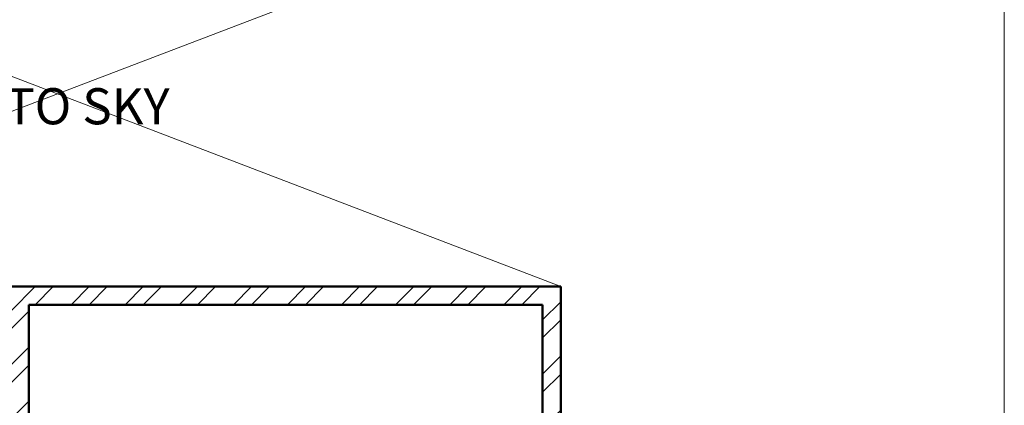
# Model space of a CAD drawing. Units: inches. Extents: x 1901 to 2863, y 888 to 2433.
# Tile 48 of 91: x 2618 to 2863, y 1636 to 1732. Entities that reach past the tile are written whole.
import ezdxf

# ---------------------------------------------------------------- set-up
doc = ezdxf.new("R2010")
doc.units = ezdxf.units.IN
for name, color, linetype, lineweight in [('A-ANNO-SYMB', 8, 'Continuous', 13), ('A-AREA-IDEN', 7, 'Continuous', 18), ('A-FLOR-FIXT', 9, 'Continuous', 18), ('A-WALL', 7, 'Continuous', 50), ('A-WALL-PATT', 8, 'Continuous', 13)]:
    doc.layers.add(name, color=color, linetype=linetype, lineweight=lineweight)
doc.styles.get("Standard").update_dxf_attribs({"font": 'arial.ttf'})

msp = doc.modelspace()

# ---------------------------------------------------------------- hatches: boundary and pattern name
at = {"layer": 'A-WALL-PATT'}
h = msp.add_hatch(dxfattribs=at)
h.set_pattern_fill('ANSI32', color=256)
h.paths.add_polyline_path([(2192.5, 2274.13), (2141.26, 2274.13), (2141.26, 2269.63), (2192.5, 2269.63)])
h.paths.add_polyline_path([(2259.93, 2274.13), (2216.5, 2274.13), (2216.5, 2269.63), (2255.43, 2269.63), (2255.43, 2214.63), (2250.81, 2214.63), (2250.81, 2210.13), (2259.93, 2210.13), (2259.93, 2215.13), (2271.76, 2215.13), (2271.76, 2217.38), (2271.76, 2219.63), (2259.93, 2219.63)])
h.paths.add_polyline_path([(2171.43, 2269.63), (2166.93, 2269.63), (2166.93, 2219.63), (2121.24, 2219.63), (2121.24, 2215.13), (2166.93, 2215.13), (2166.93, 2083.13), (2161.81, 2083.13), (2161.81, 2078.63), (2171.43, 2078.63), (2177, 2078.63), (2177, 2080.88), (2177, 2083.13), (2171.43, 2083.13), (2171.43, 2210.13), (2230.91, 2210.13), (2230.91, 2212.38), (2230.91, 2214.63), (2171.43, 2214.63)])
h.paths.add_polyline_path([(2117.26, 2274.13), (2089.43, 2274.13), (2089.43, 2219.63), (2081.14, 2219.63), (2081.14, 2215.13), (2089.43, 2215.13), (2098, 2215.13), (2098, 2217.38), (2098, 2219.63), (2093.93, 2219.63), (2093.93, 2269.63), (2117.26, 2269.63), (2117.26, 2271.88)])
h.paths.add_polyline_path([(2343.43, 2219.63), (2329.29, 2219.63), (2329.29, 2215.13), (2338.93, 2215.13), (2338.93, 2184.74), (2343.43, 2184.74)])
h.paths.add_polyline_path([(2338.93, 2083.13), (2329.29, 2083.13), (2208.97, 2083.13), (2208.97, 2078.63), (2338.93, 2078.63)])
h.paths.add_polyline_path([(2343.43, 2136.74), (2338.93, 2136.74), (2338.93, 1872.63), (2343.43, 1872.63)])
h.paths.add_polyline_path([(2343.43, 1863.63), (2397.68, 1863.63), (2397.68, 1821.63), (2384.14, 1821.63), (2384.14, 1812.63), (2418.33, 1812.63), (2418.33, 1817.13), (2418.33, 1821.63), (2406.68, 1821.63), (2406.68, 1863.63), (2459.5, 1863.63), (2459.5, 1821.63), (2447.14, 1821.63), (2447.14, 1812.63), (2459.5, 1812.63), (2468.5, 1812.63), (2468.5, 1872.63), (2394.43, 1872.63), (2334.43, 1872.63), (2334.43, 1812.63), (2343.43, 1812.63), (2353.25, 1812.63), (2353.25, 1821.63), (2343.43, 1821.63)])
h.paths.add_polyline_path([(2510.01, 1872.63), (2468.5, 1872.63), (2468.5, 1868.13), (2510.01, 1868.13)])
h.paths.add_polyline_path([(2514.01, 1817.13), (2468.5, 1817.13), (2468.5, 1812.63), (2482.11, 1812.63), (2482.11, 1800.61), (2486.61, 1800.61), (2486.61, 1812.63), (2514.01, 1812.63)])
h.paths.add_polyline_path([(2299.25, 1814.88), (2299.25, 1817.13), (2295.93, 1817.13), (2295.93, 1854.17), (2293.68, 1854.17), (2291.43, 1854.17), (2291.43, 1817.13), (2266.11, 1817.13), (2266.11, 1812.63), (2299.25, 1812.63)])
h.paths.add_polyline_path([(2218.11, 1817.13), (2206.46, 1817.13), (2171.43, 1817.13), (2171.43, 1949.13), (2190.1, 1949.13), (2190.1, 1953.63), (2163.47, 1953.63), (2163.47, 1949.13), (2166.93, 1949.13), (2166.93, 1817.13), (2114.3, 1817.13), (2114.3, 1812.63), (2218.11, 1812.63)])
h.paths.add_polyline_path([(2029.43, 1970.92), (2024.93, 1970.92), (2024.93, 1912.72), (2029.43, 1912.72)])
h.paths.add_polyline_path([(2132.3, 1953.63), (2113.93, 1953.63), (2113.93, 1975.89), (2111.68, 1975.89), (2109.43, 1975.89), (2109.43, 1953.63), (2029.43, 1953.63), (2029.43, 1949.13), (2132.3, 1949.13)])
h.paths.add_polyline_path([(2029.43, 1853.61), (2029.31, 1853.61), (2029.31, 1853.61), (2029.43, 1853.61), (2029.43, 1864.72), (2024.93, 1864.72), (2024.93, 1812.63), (2066.3, 1812.63), (2066.3, 1814.88), (2066.3, 1817.13), (2029.43, 1817.13)])
h.paths.add_polyline_path([(2122.93, 2010.09), (2120.68, 2010.09), (2118.43, 2010.09), (2118.43, 2006.13), (2029.43, 2006.13), (2029.43, 2001.63), (2109.43, 2001.63), (2109.43, 1998.04), (2113.93, 1998.04), (2113.93, 2001.63), (2122.93, 2001.63)])
h.paths.add_polyline_path([(2029.43, 2031.38), (2024.93, 2031.38), (2024.93, 1994.92), (2027.18, 1994.92), (2029.43, 1994.92)])
h.paths.add_polyline_path([(2029.43, 2136.74), (2024.93, 2136.74), (2024.93, 2067.38), (2027.18, 2067.38), (2029.43, 2067.38)])
h.paths.add_polyline_path([(2125.62, 2083.13), (2029.43, 2083.13), (2029.43, 2078.63), (2118.43, 2078.63), (2118.43, 2030.71), (2122.93, 2030.71), (2122.93, 2078.63), (2125.62, 2078.63)])
h.paths.add_polyline_path([(2029.43, 2215.13), (2040.47, 2215.13), (2040.47, 2217.38), (2040.47, 2219.63), (2024.93, 2219.63), (2024.93, 2184.74), (2029.43, 2184.74), (2029.43, 2187.78)])
h.paths.add_polyline_path([(2686.43, 2274.13), (2659.28, 2274.13), (2659.28, 2269.63), (2681.93, 2269.63), (2681.93, 2219.63), (2676.82, 2219.63), (2676.82, 2215.13), (2681.93, 2215.13), (2697.01, 2215.13), (2697.01, 2217.38), (2697.01, 2219.63), (2686.43, 2219.63)])
h.paths.add_polyline_path([(2609.93, 2269.63), (2635.28, 2269.63), (2635.28, 2274.13), (2571.43, 2274.13), (2571.43, 2269.63), (2605.43, 2269.63), (2605.43, 2214.63), (2549.1, 2214.63), (2549.1, 2210.13), (2605.43, 2210.13), (2605.43, 2083.13), (2601.01, 2083.13), (2601.01, 2080.88), (2601.01, 2078.63), (2609.93, 2078.63), (2616.16, 2078.63), (2616.16, 2080.88), (2616.16, 2083.13), (2609.93, 2083.13), (2609.93, 2215.13), (2651.46, 2215.13), (2651.46, 2217.38), (2651.46, 2219.63), (2609.93, 2219.63)])
h.paths.add_polyline_path([(2521.43, 2269.63), (2547.43, 2269.63), (2547.43, 2271.88), (2547.43, 2274.13), (2516.93, 2274.13), (2516.93, 2219.63), (2506.41, 2219.63), (2506.41, 2215.13), (2516.93, 2215.13), (2516.93, 2210.13), (2525.4, 2210.13), (2525.4, 2212.38), (2525.4, 2214.63), (2521.43, 2214.63)])
h.paths.add_polyline_path([(2456.01, 2219.63), (2439.43, 2219.63), (2439.43, 2187.89), (2443.93, 2187.89), (2443.93, 2215.13), (2456.01, 2215.13)])
h.paths.add_polyline_path([(2752.93, 2219.63), (2739.48, 2219.63), (2739.48, 2215.13), (2748.43, 2215.13), (2748.43, 2187.89), (2752.93, 2187.89)])
h.paths.add_polyline_path([(2752.93, 2139.89), (2748.43, 2139.89), (2748.43, 2083.13), (2648.42, 2083.13), (2648.42, 2078.63), (2654.93, 2078.63), (2654.93, 2039.44), (2659.43, 2039.44), (2659.43, 2078.63), (2748.43, 2078.63), (2748.43, 2063.43), (2752.93, 2063.43)])
h.paths.add_polyline_path([(2752.93, 2010.63), (2659.43, 2010.63), (2659.43, 2015.65), (2654.93, 2015.65), (2654.93, 2010.63), (2605.43, 2010.63), (2605.43, 1920.97), (2609.93, 1920.97), (2609.93, 2006.13), (2748.43, 2006.13), (2748.43, 1982.47), (2752.93, 1982.47)])
h.paths.add_polyline_path([(2752.93, 2027.43), (2748.43, 2027.43), (2748.43, 2010.63), (2752.93, 2010.63)])
h.paths.add_polyline_path([(2748.43, 1886.13), (2609.93, 1886.13), (2609.93, 1889.72), (2605.43, 1889.72), (2605.43, 1861.26), (2609.93, 1861.26), (2609.93, 1881.63), (2748.43, 1881.63)])
h.paths.add_polyline_path([(2456.86, 2228.83), (2498.4, 2228.83), (2498.4, 2247.49), (2456.86, 2247.49)], flags=9)
h.paths.add_polyline_path([(2038.6, 2237.42), (2080.17, 2237.42), (2080.17, 2256.08), (2038.6, 2256.08)], flags=9)
h.paths.add_polyline_path([(2292.01, 1062.39), (2539.93, 1062.39), (2539.93, 1099.49), (2292.01, 1099.49)], flags=9)
h.paths.add_polyline_path([(2424.91, 1832.25), (2448.51, 1832.25), (2448.51, 1846.68), (2424.91, 1846.68)], flags=25)
h.paths.add_polyline_path([(2359.08, 1832.25), (2382.68, 1832.25), (2382.68, 1846.68), (2359.08, 1846.68)], flags=25)
h.paths.add_polyline_path([(2352.9, 1684.8), (2367.54, 1684.8), (2367.54, 1697.17), (2352.9, 1697.17)], flags=9)
h.paths.add_polyline_path([(2079.29, 1755.83), (2169.02, 1755.83), (2169.02, 1774.37), (2079.29, 1774.37)], flags=9)
h.paths.add_polyline_path([(2404.09, 1373.86), (2404.09, 1463.59), (2385.54, 1463.59), (2385.54, 1373.86)], flags=9)
h.paths.add_polyline_path([(2268.09, 2236.37), (2309.64, 2236.37), (2309.64, 2255.03), (2268.09, 2255.03)], flags=9)
h.paths.add_polyline_path([(2575.96, 1700.95), (2665.7, 1700.95), (2665.7, 1719.5), (2575.96, 1719.5)], flags=9)
h.paths.add_polyline_path([(2302.96, 1878.47), (2329.52, 1878.47), (2329.52, 1888.78), (2302.96, 1888.78)], flags=9)
h.paths.add_polyline_path([(2097.42, 2240.58), (2126.57, 2240.58), (2126.57, 2259.23), (2097.42, 2259.23)], flags=9)
h.paths.add_polyline_path([(2208.72, 2246.12), (2237.88, 2246.12), (2237.88, 2264.78), (2208.72, 2264.78)], flags=9)
h.paths.add_polyline_path([(2038.15, 1925.96), (2076.99, 1925.96), (2076.99, 1944.62), (2038.15, 1944.62)], flags=9)
h.paths.add_polyline_path([(2239.14, 1926.67), (2288.46, 1926.67), (2288.46, 1945.33), (2239.14, 1945.33)], flags=9)
h.paths.add_polyline_path([(2175.43, 2007.33), (2212.36, 2007.33), (2212.36, 2025.99), (2175.43, 2025.99)], flags=9)
h.paths.add_polyline_path([(2225.03, 2091.79), (2263.87, 2091.79), (2263.87, 2110.45), (2225.03, 2110.45)], flags=9)
h.paths.add_polyline_path([(2035.4, 2098.48), (2074.24, 2098.48), (2074.24, 2117.14), (2035.4, 2117.14)], flags=9)
h.paths.add_polyline_path([(2050.1, 2029.21), (2083.26, 2029.21), (2083.26, 2047.87), (2050.1, 2047.87)], flags=9)
h.paths.add_polyline_path([(2069.68, 1956.72), (2098.83, 1956.72), (2098.83, 1975.38), (2069.68, 1975.38)], flags=25)
h.paths.add_polyline_path([(2328.62, 1753.34), (2361.66, 1753.34), (2361.66, 1771.99), (2328.62, 1771.99)], flags=9)
h.paths.add_polyline_path([(2395.16, 2060.89), (2395.16, 2140.65), (2378.68, 2140.65), (2378.68, 2060.89)], flags=9)
h.paths.add_polyline_path([(2463.73, 2059.02), (2492.89, 2059.02), (2492.89, 2077.68), (2463.73, 2077.68)], flags=9)
h.paths.add_polyline_path([(2458.03, 2181.54), (2496.87, 2181.54), (2496.87, 2200.19), (2458.03, 2200.19)], flags=9)
h.paths.add_polyline_path([(2527.58, 2243.07), (2556.73, 2243.07), (2556.73, 2261.73), (2527.58, 2261.73)], flags=9)
h.paths.add_polyline_path([(2694.46, 2232.77), (2736.03, 2232.77), (2736.03, 2251.42), (2694.46, 2251.42)], flags=9)
h.paths.add_polyline_path([(2637.82, 2249.22), (2666.98, 2249.22), (2666.98, 2267.88), (2637.82, 2267.88)], flags=9)
h.paths.add_polyline_path([(2623.69, 2183.54), (2662.53, 2183.54), (2662.53, 2202.2), (2623.69, 2202.2)], flags=9)
h.paths.add_polyline_path([(2691.97, 2021.5), (2725.12, 2021.5), (2725.12, 2040.16), (2691.97, 2040.16)], flags=9)
h.paths.add_polyline_path([(2621.04, 1975.91), (2662.34, 1975.91), (2662.34, 1994.57), (2621.04, 1994.57)], flags=25)
h.paths.add_polyline_path([(2479.03, 1927.62), (2519.84, 1927.62), (2519.84, 1946.28), (2479.03, 1946.28)], flags=9)
h.paths.add_polyline_path([(2670.94, 1849.08), (2716.01, 1849.08), (2716.01, 1867.73), (2670.94, 1867.73)], flags=9)
h.paths.add_polyline_path([(2523.61, 1782.96), (2550.17, 1782.96), (2550.17, 1793.26), (2523.61, 1793.26)], flags=9)
h.paths.add_polyline_path([(2450.84, 1207.33), (2492.39, 1207.33), (2492.39, 1225.99), (2450.84, 1225.99)], flags=9)
h.paths.add_polyline_path([(2527.75, 1203.84), (2556.91, 1203.84), (2556.91, 1222.5), (2527.75, 1222.5)], flags=9)
h.paths.add_polyline_path([(2639.11, 1207.2), (2668.27, 1207.2), (2668.27, 1225.86), (2639.11, 1225.86)], flags=9)
h.paths.add_polyline_path([(2692.59, 1218.97), (2734.17, 1218.97), (2734.17, 1237.62), (2692.59, 1237.62)], flags=9)
h.paths.add_polyline_path([(2669.27, 1366.33), (2708.11, 1366.33), (2708.11, 1384.99), (2669.27, 1384.99)], flags=9)
h.paths.add_polyline_path([(2463.31, 1358.03), (2502.15, 1358.03), (2502.15, 1376.69), (2463.31, 1376.69)], flags=9)
h.paths.add_polyline_path([(2494.72, 1449.96), (2531.65, 1449.96), (2531.65, 1468.62), (2494.72, 1468.62)], flags=9)
h.paths.add_polyline_path([(2675.57, 1422.16), (2708.72, 1422.16), (2708.72, 1440.81), (2675.57, 1440.81)], flags=9)
h.paths.add_polyline_path([(2685.63, 1493.89), (2714.79, 1493.89), (2714.79, 1512.55), (2685.63, 1512.55)], flags=9)
h.paths.add_polyline_path([(2686.8, 1529.91), (2725.65, 1529.91), (2725.65, 1548.57), (2686.8, 1548.57)], flags=9)
h.paths.add_polyline_path([(2503.65, 1537.99), (2552.97, 1537.99), (2552.97, 1556.65), (2503.65, 1556.65)], flags=9)
h.paths.add_polyline_path([(2291.71, 1643.5), (2318.28, 1643.5), (2318.28, 1653.81), (2291.71, 1653.81)], flags=9)
h.paths.add_polyline_path([(2450.63, 1610.52), (2477.19, 1610.52), (2477.19, 1620.82), (2450.63, 1620.82)], flags=9)
h.paths.add_polyline_path([(2359.99, 1551.81), (2422.25, 1551.81), (2422.25, 1562.12), (2359.99, 1562.12)], flags=9)
h.paths.add_polyline_path([(2280.11, 1249.01), (2321.65, 1249.01), (2321.65, 1267.66), (2280.11, 1267.66)], flags=9)
h.paths.add_polyline_path([(2164.06, 1274.23), (2193.22, 1274.23), (2193.22, 1292.89), (2164.06, 1292.89)], flags=9)
h.paths.add_polyline_path([(2118.21, 1277.69), (2151.25, 1277.69), (2151.25, 1296.35), (2118.21, 1296.35)], flags=9)
h.paths.add_polyline_path([(2031.95, 1268.53), (2073.52, 1268.53), (2073.52, 1287.19), (2031.95, 1287.19)], flags=9)
h.paths.add_polyline_path([(2050.2, 1409.08), (2089.04, 1409.08), (2089.04, 1427.74), (2050.2, 1427.74)], flags=9)
h.paths.add_polyline_path([(2243.74, 1421.03), (2282.58, 1421.03), (2282.58, 1439.69), (2243.74, 1439.69)], flags=9)
h.paths.add_polyline_path([(2190.75, 1509.77), (2231.56, 1509.77), (2231.56, 1528.43), (2190.75, 1528.43)], flags=9)
h.paths.add_polyline_path([(2058.39, 1475.42), (2091.55, 1475.42), (2091.55, 1494.07), (2058.39, 1494.07)], flags=9)
h.paths.add_polyline_path([(2062.45, 1553.09), (2091.6, 1553.09), (2091.6, 1571.75), (2062.45, 1571.75)], flags=9)
h.paths.add_polyline_path([(2219.52, 1590.37), (2266.15, 1590.37), (2266.15, 1609.02), (2219.52, 1609.02)], flags=9)
h.paths.add_polyline_path([(2041.07, 1584.19), (2079.91, 1584.19), (2079.91, 1602.85), (2041.07, 1602.85)], flags=9)
h = msp.add_hatch(dxfattribs=at)
h.set_pattern_fill('ANSI32', color=256)
h.paths.add_polyline_path([(2443.93, 2139.89), (2439.43, 2139.89), (2439.43, 2069.35), (2441.68, 2069.35), (2443.93, 2069.35), (2443.93, 2078.63), (2521.93, 2078.63), (2521.93, 2075.07), (2524.18, 2075.07), (2526.43, 2075.07), (2526.43, 2078.63), (2571.75, 2078.63), (2571.75, 2080.88), (2571.75, 2083.13), (2443.93, 2083.13)])
h.paths.add_polyline_path([(2526.43, 2054.63), (2524.18, 2054.63), (2521.93, 2054.63), (2521.93, 2030.63), (2443.93, 2030.63), (2443.93, 2045.35), (2439.43, 2045.35), (2439.43, 1983.87), (2443.93, 1983.87), (2443.93, 2026.13), (2521.93, 2026.13), (2526.43, 2026.13)])
h.paths.add_polyline_path([(2443.93, 1923.87), (2439.43, 1923.87), (2439.43, 1872.63), (2443.93, 1872.63)])
h.paths.add_polyline_path([(2636.23, 1766.13), (2609.93, 1766.13), (2609.93, 1779.79), (2605.43, 1779.79), (2605.43, 1766.13), (2486.61, 1766.13), (2486.61, 1770.67), (2482.11, 1770.67), (2482.11, 1766.13), (2482.11, 1761.63), (2636.23, 1761.63), (2636.23, 1763.88)])
h.paths.add_polyline_path([(2519.54, 1663.38), (2519.54, 1665.63), (2494.93, 1665.63), (2481.83, 1665.63), (2481.83, 1663.38), (2481.83, 1661.13), (2490.43, 1661.13), (2490.43, 1640.16), (2494.93, 1640.16), (2494.93, 1661.13), (2519.54, 1661.13)])
h.paths.add_polyline_path([(2443.93, 1712.13), (2443.93, 1716.63), (2414.46, 1716.63), (2414.46, 1712.13), (2439.43, 1712.13), (2439.43, 1545.51), (2443.93, 1545.51), (2443.93, 1661.13), (2448.47, 1661.13), (2448.47, 1665.63), (2443.93, 1665.63)])
h.paths.add_polyline_path([(2343.43, 1712.13), (2365.52, 1712.13), (2365.52, 1714.38), (2365.52, 1716.63), (2333.87, 1716.63), (2333.87, 1714.38), (2333.87, 1712.13), (2338.93, 1712.13), (2338.93, 1575.63), (2338.93, 1545.51), (2343.43, 1545.51), (2343.43, 1547.51), (2343.43, 1580.13)])
h.paths.add_polyline_path([(2752.93, 1665.63), (2579.54, 1665.63), (2579.54, 1661.13), (2615.93, 1661.13), (2615.93, 1529.13), (2598.93, 1529.13), (2598.93, 1524.63), (2623.13, 1524.63), (2623.13, 1526.88), (2623.13, 1529.13), (2620.43, 1529.13), (2620.43, 1661.13), (2748.43, 1661.13), (2748.43, 1633.5), (2752.93, 1633.5)])
h.paths.add_polyline_path([(2752.93, 1419.93), (2748.43, 1419.93), (2748.43, 1400.13), (2659.43, 1400.13), (2659.43, 1444.33), (2657.18, 1444.33), (2654.93, 1444.33), (2654.93, 1400.13), (2643.65, 1400.13), (2643.65, 1395.63), (2748.43, 1395.63), (2748.43, 1364.04), (2752.93, 1364.04)])
h.paths.add_polyline_path([(2752.93, 1492.88), (2748.43, 1492.88), (2748.43, 1476.63), (2667.43, 1476.63), (2667.43, 1479.71), (2665.18, 1479.71), (2662.93, 1479.71), (2662.93, 1476.63), (2654.93, 1476.63), (2654.93, 1469.54), (2659.43, 1469.54), (2659.43, 1472.13), (2748.43, 1472.13), (2748.43, 1455.93), (2752.93, 1455.93)])
h.paths.add_polyline_path([(2752.93, 1304.04), (2748.43, 1304.04), (2748.43, 1263.63), (2738.66, 1263.63), (2738.66, 1259.13), (2752.93, 1259.13)])
h.paths.add_polyline_path([(2685.93, 1259.13), (2695.49, 1259.13), (2695.49, 1261.38), (2695.49, 1263.63), (2677.84, 1263.63), (2677.84, 1261.38), (2677.84, 1259.13), (2681.43, 1259.13), (2681.43, 1203.63), (2653.28, 1203.63), (2653.28, 1199.13), (2685.93, 1199.13), (2685.93, 1203.63)])
h.paths.add_polyline_path([(2609.43, 1395.63), (2611.85, 1395.63), (2611.85, 1400.13), (2598.89, 1400.13), (2598.89, 1397.88), (2598.89, 1395.63), (2604.93, 1395.63), (2604.93, 1268.13), (2554.73, 1268.13), (2554.73, 1265.88), (2554.73, 1263.63), (2604.93, 1263.63), (2604.93, 1203.63), (2571.31, 1203.63), (2571.31, 1199.13), (2604.93, 1199.13), (2629.28, 1199.13), (2629.28, 1201.38), (2629.28, 1203.63), (2609.43, 1203.63), (2609.43, 1258.63), (2609.43, 1259.13), (2654.8, 1259.13), (2654.8, 1263.63), (2609.43, 1263.63)])
h.paths.add_polyline_path([(2443.93, 1304.04), (2439.43, 1304.04), (2439.43, 1259.13), (2443.93, 1259.13), (2456.16, 1259.13), (2456.16, 1261.38), (2456.16, 1263.63), (2443.93, 1263.63)])
h.paths.add_polyline_path([(2525.43, 1263.63), (2531.78, 1263.63), (2531.78, 1268.13), (2520.93, 1268.13), (2520.93, 1263.63), (2511.41, 1263.63), (2511.41, 1259.13), (2520.93, 1259.13), (2520.93, 1199.13), (2547.31, 1199.13), (2547.31, 1201.38), (2547.31, 1203.63), (2525.43, 1203.63)])
h.paths.add_polyline_path([(2443.93, 1434.84), (2439.43, 1434.84), (2439.43, 1364.04), (2441.68, 1364.04), (2443.93, 1364.04)])
h.paths.add_polyline_path([(2567.13, 1400.13), (2443.93, 1400.13), (2443.93, 1395.63), (2567.13, 1395.63)])
h.paths.add_polyline_path([(2443.93, 1545.51), (2439.43, 1545.51), (2439.43, 1494.84), (2443.93, 1494.84)])
h.paths.add_polyline_path([(2494.93, 1553.35), (2492.68, 1553.35), (2490.43, 1553.35), (2490.43, 1524.63), (2494.93, 1524.63), (2525.94, 1524.63), (2525.94, 1526.88), (2525.94, 1529.13), (2494.93, 1529.13)])
h.paths.add_polyline_path([(2752.93, 1573.5), (2748.43, 1573.5), (2748.43, 1529.13), (2657.76, 1529.13), (2657.76, 1524.63), (2662.93, 1524.63), (2662.93, 1498.63), (2667.43, 1498.63), (2667.43, 1524.63), (2748.43, 1524.63), (2748.43, 1516.88), (2752.93, 1516.88)])
h.paths.add_polyline_path([(2038.6, 2237.42), (2080.17, 2237.42), (2080.17, 2256.08), (2038.6, 2256.08)], flags=9)
h.paths.add_polyline_path([(2292.01, 1062.39), (2539.93, 1062.39), (2539.93, 1099.49), (2292.01, 1099.49)], flags=9)
h.paths.add_polyline_path([(2424.91, 1832.25), (2448.51, 1832.25), (2448.51, 1846.68), (2424.91, 1846.68)], flags=9)
h.paths.add_polyline_path([(2359.08, 1832.25), (2382.68, 1832.25), (2382.68, 1846.68), (2359.08, 1846.68)], flags=9)
h.paths.add_polyline_path([(2352.9, 1684.8), (2367.54, 1684.8), (2367.54, 1697.17), (2352.9, 1697.17)], flags=9)
h.paths.add_polyline_path([(2079.29, 1755.83), (2169.02, 1755.83), (2169.02, 1774.37), (2079.29, 1774.37)], flags=9)
h.paths.add_polyline_path([(2404.09, 1373.86), (2404.09, 1463.59), (2385.54, 1463.59), (2385.54, 1373.86)], flags=9)
h.paths.add_polyline_path([(2268.09, 2236.37), (2309.64, 2236.37), (2309.64, 2255.03), (2268.09, 2255.03)], flags=9)
h.paths.add_polyline_path([(2575.96, 1700.95), (2665.7, 1700.95), (2665.7, 1719.5), (2575.96, 1719.5)], flags=9)
h.paths.add_polyline_path([(2302.96, 1878.47), (2329.52, 1878.47), (2329.52, 1888.78), (2302.96, 1888.78)], flags=9)
h.paths.add_polyline_path([(2097.42, 2240.58), (2126.57, 2240.58), (2126.57, 2259.23), (2097.42, 2259.23)], flags=9)
h.paths.add_polyline_path([(2208.72, 2246.12), (2237.88, 2246.12), (2237.88, 2264.78), (2208.72, 2264.78)], flags=9)
h.paths.add_polyline_path([(2038.15, 1925.96), (2076.99, 1925.96), (2076.99, 1944.62), (2038.15, 1944.62)], flags=9)
h.paths.add_polyline_path([(2239.14, 1926.67), (2288.46, 1926.67), (2288.46, 1945.33), (2239.14, 1945.33)], flags=9)
h.paths.add_polyline_path([(2175.43, 2007.33), (2212.36, 2007.33), (2212.36, 2025.99), (2175.43, 2025.99)], flags=9)
h.paths.add_polyline_path([(2225.03, 2091.79), (2263.87, 2091.79), (2263.87, 2110.45), (2225.03, 2110.45)], flags=9)
h.paths.add_polyline_path([(2035.4, 2098.48), (2074.24, 2098.48), (2074.24, 2117.14), (2035.4, 2117.14)], flags=9)
h.paths.add_polyline_path([(2050.1, 2029.21), (2083.26, 2029.21), (2083.26, 2047.87), (2050.1, 2047.87)], flags=9)
h.paths.add_polyline_path([(2069.68, 1956.72), (2098.83, 1956.72), (2098.83, 1975.38), (2069.68, 1975.38)], flags=9)
h.paths.add_polyline_path([(2328.62, 1753.34), (2361.66, 1753.34), (2361.66, 1771.99), (2328.62, 1771.99)], flags=9)
h.paths.add_polyline_path([(2395.16, 2060.89), (2395.16, 2140.65), (2378.68, 2140.65), (2378.68, 2060.89)], flags=9)
h.paths.add_polyline_path([(2463.73, 2059.02), (2492.89, 2059.02), (2492.89, 2077.68), (2463.73, 2077.68)], flags=9)
h.paths.add_polyline_path([(2458.03, 2181.54), (2496.87, 2181.54), (2496.87, 2200.19), (2458.03, 2200.19)], flags=9)
h.paths.add_polyline_path([(2456.86, 2228.83), (2498.4, 2228.83), (2498.4, 2247.49), (2456.86, 2247.49)], flags=9)
h.paths.add_polyline_path([(2527.58, 2243.07), (2556.73, 2243.07), (2556.73, 2261.73), (2527.58, 2261.73)], flags=9)
h.paths.add_polyline_path([(2694.46, 2232.77), (2736.03, 2232.77), (2736.03, 2251.42), (2694.46, 2251.42)], flags=9)
h.paths.add_polyline_path([(2637.82, 2249.22), (2666.98, 2249.22), (2666.98, 2267.88), (2637.82, 2267.88)], flags=9)
h.paths.add_polyline_path([(2623.69, 2183.54), (2662.53, 2183.54), (2662.53, 2202.2), (2623.69, 2202.2)], flags=9)
h.paths.add_polyline_path([(2691.97, 2021.5), (2725.12, 2021.5), (2725.12, 2040.16), (2691.97, 2040.16)], flags=9)
h.paths.add_polyline_path([(2621.04, 1975.91), (2662.34, 1975.91), (2662.34, 1994.57), (2621.04, 1994.57)], flags=9)
h.paths.add_polyline_path([(2479.03, 1927.62), (2519.84, 1927.62), (2519.84, 1946.28), (2479.03, 1946.28)], flags=9)
h.paths.add_polyline_path([(2670.94, 1849.08), (2716.01, 1849.08), (2716.01, 1867.73), (2670.94, 1867.73)], flags=9)
h.paths.add_polyline_path([(2523.61, 1782.96), (2550.17, 1782.96), (2550.17, 1793.26), (2523.61, 1793.26)], flags=9)
h.paths.add_polyline_path([(2450.84, 1207.33), (2492.39, 1207.33), (2492.39, 1225.99), (2450.84, 1225.99)], flags=9)
h.paths.add_polyline_path([(2527.75, 1203.84), (2556.91, 1203.84), (2556.91, 1222.5), (2527.75, 1222.5)], flags=9)
h.paths.add_polyline_path([(2639.11, 1207.2), (2668.27, 1207.2), (2668.27, 1225.86), (2639.11, 1225.86)], flags=9)
h.paths.add_polyline_path([(2692.59, 1218.97), (2734.17, 1218.97), (2734.17, 1237.62), (2692.59, 1237.62)], flags=9)
h.paths.add_polyline_path([(2669.27, 1366.33), (2708.11, 1366.33), (2708.11, 1384.99), (2669.27, 1384.99)], flags=25)
h.paths.add_polyline_path([(2463.31, 1358.03), (2502.15, 1358.03), (2502.15, 1376.69), (2463.31, 1376.69)], flags=9)
h.paths.add_polyline_path([(2494.72, 1449.96), (2531.65, 1449.96), (2531.65, 1468.62), (2494.72, 1468.62)], flags=9)
h.paths.add_polyline_path([(2675.57, 1422.16), (2708.72, 1422.16), (2708.72, 1440.81), (2675.57, 1440.81)], flags=25)
h.paths.add_polyline_path([(2685.63, 1493.89), (2714.79, 1493.89), (2714.79, 1512.55), (2685.63, 1512.55)], flags=9)
h.paths.add_polyline_path([(2686.8, 1529.91), (2725.65, 1529.91), (2725.65, 1548.57), (2686.8, 1548.57)], flags=25)
h.paths.add_polyline_path([(2503.65, 1537.99), (2552.97, 1537.99), (2552.97, 1556.65), (2503.65, 1556.65)], flags=9)
h.paths.add_polyline_path([(2291.71, 1643.5), (2318.28, 1643.5), (2318.28, 1653.81), (2291.71, 1653.81)], flags=9)
h.paths.add_polyline_path([(2450.63, 1610.52), (2477.19, 1610.52), (2477.19, 1620.82), (2450.63, 1620.82)], flags=9)
h.paths.add_polyline_path([(2359.99, 1551.81), (2422.25, 1551.81), (2422.25, 1562.12), (2359.99, 1562.12)], flags=9)
h.paths.add_polyline_path([(2280.11, 1249.01), (2321.65, 1249.01), (2321.65, 1267.66), (2280.11, 1267.66)], flags=9)
h.paths.add_polyline_path([(2164.06, 1274.23), (2193.22, 1274.23), (2193.22, 1292.89), (2164.06, 1292.89)], flags=9)
h.paths.add_polyline_path([(2118.21, 1277.69), (2151.25, 1277.69), (2151.25, 1296.35), (2118.21, 1296.35)], flags=9)
h.paths.add_polyline_path([(2031.95, 1268.53), (2073.52, 1268.53), (2073.52, 1287.19), (2031.95, 1287.19)], flags=9)
h.paths.add_polyline_path([(2050.2, 1409.08), (2089.04, 1409.08), (2089.04, 1427.74), (2050.2, 1427.74)], flags=9)
h.paths.add_polyline_path([(2243.74, 1421.03), (2282.58, 1421.03), (2282.58, 1439.69), (2243.74, 1439.69)], flags=9)
h.paths.add_polyline_path([(2190.75, 1509.77), (2231.56, 1509.77), (2231.56, 1528.43), (2190.75, 1528.43)], flags=9)
h.paths.add_polyline_path([(2058.39, 1475.42), (2091.55, 1475.42), (2091.55, 1494.07), (2058.39, 1494.07)], flags=9)
h.paths.add_polyline_path([(2062.45, 1553.09), (2091.6, 1553.09), (2091.6, 1571.75), (2062.45, 1571.75)], flags=9)
h.paths.add_polyline_path([(2219.52, 1590.37), (2266.15, 1590.37), (2266.15, 1609.02), (2219.52, 1609.02)], flags=9)
h.paths.add_polyline_path([(2041.07, 1584.19), (2079.91, 1584.19), (2079.91, 1602.85), (2041.07, 1602.85)], flags=9)

# ---------------------------------------------------------------- linework, layer by layer
at = {"layer": 'A-ANNO-SYMB'}
for p, q in [((2502.24, 1761.63), (2752.93, 1665.63)), ((2752.93, 1761.63), (2502.24, 1665.63))]:
    msp.add_line(p, q, dxfattribs=at)
at = {"layer": 'A-FLOR-FIXT'}
msp.add_lwpolyline([(1901.45, 2433.12), (2863.43, 2433.12), (2863.43, 961.82), (1901.45, 961.82)], close=True, dxfattribs=at)
at = {"layer": 'A-WALL'}
for p, q in [((2752.93, 1665.63), (2481.83, 1665.63)), ((2752.93, 1665.63), (2748.43, 1665.63)), ((2752.93, 1665.63), (2752.93, 1259.13)), ((2620.43, 1661.13), (2620.43, 1529.13)), ((2620.43, 1661.13), (2748.43, 1661.13)), ((2748.43, 1661.13), (2748.43, 1529.13))]:
    msp.add_line(p, q, dxfattribs=at)

# ---------------------------------------------------------------- texts
at = {"layer": 'A-AREA-IDEN', "insert": (2578.82, 1715.03), "char_height": 9, "attachment_point": 1}
msp.add_mtext_dynamic_manual_height_columns('OPEN TO SKY', width=233.3304, gutter_width=12.5, heights=[0], dxfattribs=at)

doc.saveas('drawing.dxf')
